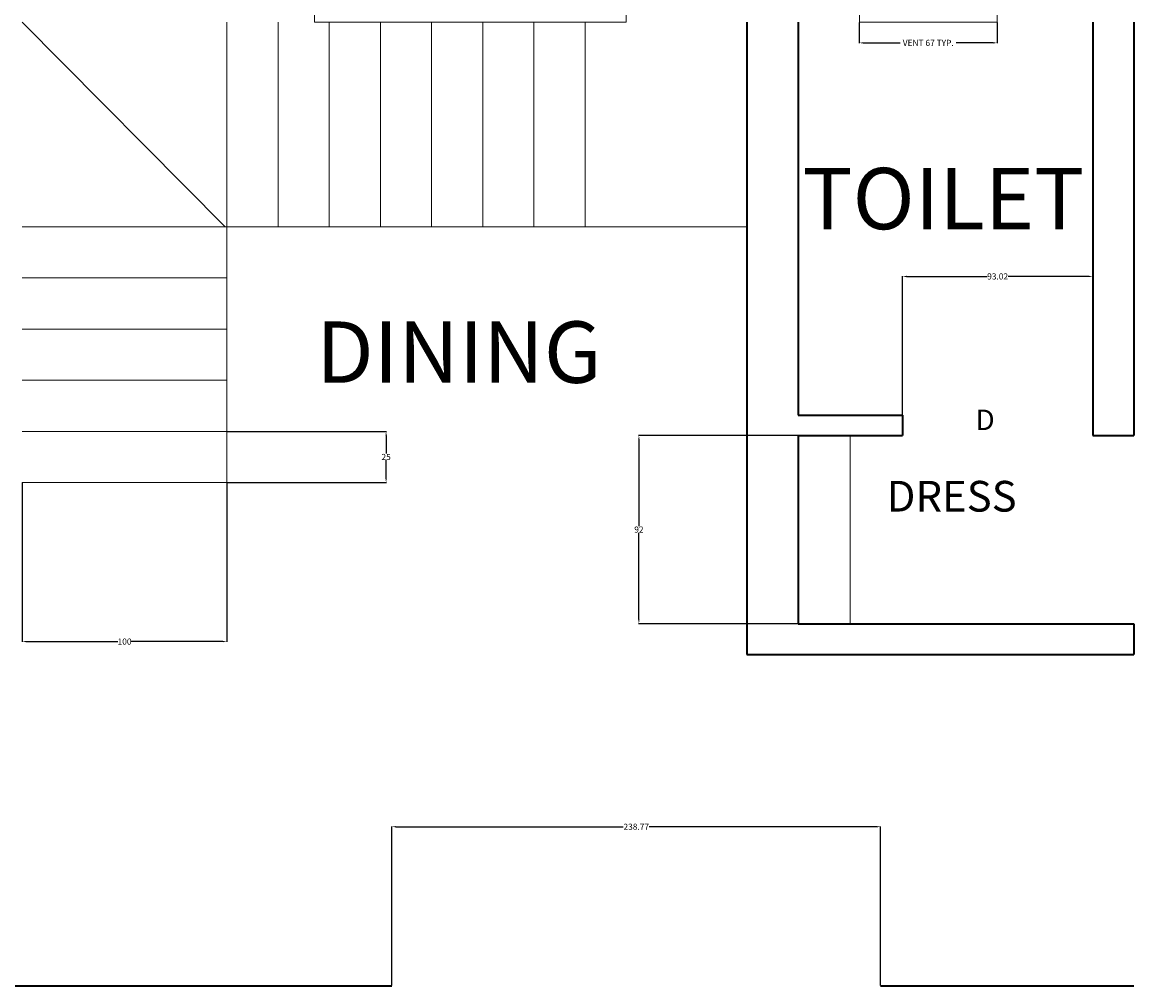
# Model space of a CAD drawing. Units: centimetres. Extents: x -121 to 3851, y -16 to 1180.
# Tile 5 of 16: x 415 to 958, y 384 to 855. Entities that reach past the tile are written whole.
import ezdxf

# ---------------------------------------------------------------- set-up
doc = ezdxf.new("R2010")
doc.units = ezdxf.units.CM
doc.header["$MEASUREMENT"] = 0
for name, color, linetype, lineweight in [('A-ANNO-DIMS', 2, 'Continuous', 18), ('A-ANNO-IDEN', 3, 'Continuous', 13), ('A-AREA-IDEN', 3, 'Continuous', 18), ('A-FLOR-CASE', 9, 'Continuous', 18), ('A-FLOR-STRS', 3, 'Continuous', 18), ('A-GLAZ', 4, 'Continuous', 18), ('A-WALL', 7, 'Continuous', 35)]:
    doc.layers.add(name, color=color, linetype=linetype, lineweight=lineweight)
doc.styles.get("Standard").update_dxf_attribs({"font": 'arial.ttf'})
doc.dimstyles.get("Standard").update_dxf_attribs({"dimtxt": 3, "dimasz": 2, "dimexe": 0.18, "dimexo": 0.0625, "dimgap": 0.09, "dimtad": 0, "dimtih": 1, "dimtoh": 1, "dimdec": 0, "dimzin": 0, "dimdsep": 46, "dimtxsty": 'Standard', "dimcen": 0.09, "dimadec": 0, "dimazin": 0, "dimtfac": 1, "dimtdec": 0, "dimtofl": 0, "dimtmove": 0, "dimatfit": 3, "dimfxl": 1, "dimtolj": 1, "dimtzin": 0, "dimarcsym": 0})

# ---------------------------------------------------------------- blocks, each defined once
blk = doc.blocks.new('WIN-152CM')
for p, q in [((0, 17.5), (152.19, 17.5)), ((0, 12.5), (152.19, 12.5)), ((0, 7.5), (152.19, 7.5))]:
    blk.add_line(p, q)
blk.add_lwpolyline([(0, 25), (152.19, 25), (152.19, 0), (0, 0)], close=True)
blk = doc.blocks.new('VENT-67CM')
for p, q in [((0, 15.5), (67.32, 15.5)), ((0, 12.5), (67.32, 12.5)), ((0, 9.5), (67.32, 9.5))]:
    blk.add_line(p, q)
blk.add_lwpolyline([(0, 25), (67.32, 25), (67.32, 0), (0, 0)], close=True)
blk = doc.blocks.new('STAIR-L-RETURN')
for p, q in [((0, 225), (99.13, 125)), ((100, 100), (100, 225)), ((125, 125), (125, 225)), ((150, 125), (150, 225)), ((175, 125), (175, 225)), ((200, 125), (200, 225)), ((225, 125), (225, 225)), ((250, 125), (250, 225)), ((275, 125), (275, 225)), ((0, 125), (99.13, 125)), ((99.13, 125), (354, 125)), ((100, 0), (100, 125)), ((0, 100), (100, 100)), ((0, 75), (100, 75)), ((0, 50), (100, 50)), ((0, 25), (100, 25)), ((0, 0), (100, 0))]:
    blk.add_line(p, q)
blk = doc.blocks.new('*D29')
at = {"layer": 'A-ANNO-DIMS', "color": 0, "lineweight": -2, "transparency": 16777216}
for p, q in [((823.97, 854.95), (823.97, 844.74)), ((891.29, 854.95), (891.29, 844.74)), ((825.97, 844.92), (843.99, 844.92)), ((889.29, 844.92), (871.27, 844.92))]:
    blk.add_line(p, q, dxfattribs=at)
at = {"layer": 'A-ANNO-DIMS', "color": 0, "transparency": 16777216}
for points in [[(825.97, 845.25), (825.97, 844.58), (823.97, 844.92)], [(889.29, 845.25), (889.29, 844.58), (891.29, 844.92)]]:
    blk.add_solid(points, dxfattribs=at)
at = {"layer": 'Defpoints', "color": 0, "transparency": 16777216}
for p in [(823.97, 855.01), (891.29, 855.01), (891.29, 844.92)]:
    blk.add_point(p, dxfattribs=at)
at = {"layer": 'A-ANNO-DIMS', "color": 0, "transparency": 16777216, "insert": (857.63, 844.92), "char_height": 3, "attachment_point": 5}
blk.add_mtext('\\A1;VENT 67 TYP.', dxfattribs=at)
blk = doc.blocks.new('*D45')
at = {"layer": 'A-ANNO-DIMS', "color": 0, "lineweight": -2, "transparency": 16777216}
for p, q in [((595.61, 384.08), (595.61, 461.94)), ((597.61, 461.76), (708.65, 461.76)), ((832.38, 461.76), (721.34, 461.76)), ((834.38, 384.08), (834.38, 461.94))]:
    blk.add_line(p, q, dxfattribs=at)
at = {"layer": 'A-ANNO-DIMS', "color": 0, "transparency": 16777216}
for points in [[(597.61, 462.1), (597.61, 461.43), (595.61, 461.76)], [(832.38, 462.1), (832.38, 461.43), (834.38, 461.76)]]:
    blk.add_solid(points, dxfattribs=at)
at = {"layer": 'Defpoints', "color": 0, "transparency": 16777216}
for p in [(834.38, 461.76), (595.61, 384.01), (834.38, 384.01)]:
    blk.add_point(p, dxfattribs=at)
at = {"layer": 'A-ANNO-DIMS', "color": 0, "transparency": 16777216, "insert": (715, 461.76), "char_height": 3, "attachment_point": 5}
blk.add_mtext('\\A1;238.77', dxfattribs=at)
blk = doc.blocks.new('*D56')
at = {"layer": 'A-ANNO-DIMS', "color": 0, "lineweight": -2, "transparency": 16777216}
for p, q in [((415.04, 629.95), (415.04, 552.08)), ((515.04, 629.95), (515.04, 552.08)), ((417.04, 552.26), (461.78, 552.26)), ((513.04, 552.26), (468.3, 552.26))]:
    blk.add_line(p, q, dxfattribs=at)
at = {"layer": 'A-ANNO-DIMS', "color": 0, "transparency": 16777216}
for points in [[(417.04, 552.6), (417.04, 551.93), (415.04, 552.26)], [(513.04, 552.6), (513.04, 551.93), (515.04, 552.26)]]:
    blk.add_solid(points, dxfattribs=at)
at = {"layer": 'Defpoints', "color": 0, "transparency": 16777216}
for p in [(415.04, 630.01), (515.04, 630.01), (415.04, 552.26)]:
    blk.add_point(p, dxfattribs=at)
at = {"layer": 'A-ANNO-DIMS', "color": 0, "transparency": 16777216, "insert": (465.04, 552.26), "char_height": 3, "attachment_point": 5}
blk.add_mtext('\\A1;100', dxfattribs=at)
blk = doc.blocks.new('*D57')
at = {"layer": 'A-ANNO-DIMS', "color": 0, "lineweight": -2, "transparency": 16777216}
for p, q in [((515.1, 655.01), (592.97, 655.01)), ((592.79, 653.01), (592.79, 644.14)), ((592.79, 632.01), (592.79, 640.89)), ((515.1, 630.01), (592.97, 630.01))]:
    blk.add_line(p, q, dxfattribs=at)
at = {"layer": 'A-ANNO-DIMS', "color": 0, "transparency": 16777216}
for points in [[(592.45, 653.01), (593.12, 653.01), (592.79, 655.01)], [(592.45, 632.01), (593.12, 632.01), (592.79, 630.01)]]:
    blk.add_solid(points, dxfattribs=at)
at = {"layer": 'Defpoints', "color": 0, "transparency": 16777216}
for p in [(515.04, 655.01), (515.04, 630.01), (592.79, 630.01)]:
    blk.add_point(p, dxfattribs=at)
at = {"layer": 'A-ANNO-DIMS', "color": 0, "transparency": 16777216, "insert": (592.79, 642.51), "char_height": 3, "attachment_point": 5}
blk.add_mtext('\\A1;25', dxfattribs=at)
blk = doc.blocks.new('*D58')
at = {"layer": 'A-ANNO-DIMS', "color": 0, "lineweight": -2, "transparency": 16777216}
for p, q in [((845.02, 653.08), (845.02, 730.94)), ((847.02, 730.76), (886.39, 730.76)), ((936.04, 730.76), (896.66, 730.76)), ((938.04, 653.08), (938.04, 730.94))]:
    blk.add_line(p, q, dxfattribs=at)
at = {"layer": 'A-ANNO-DIMS', "color": 0, "transparency": 16777216}
for points in [[(847.02, 731.1), (847.02, 730.43), (845.02, 730.76)], [(936.04, 731.1), (936.04, 730.43), (938.04, 730.76)]]:
    blk.add_solid(points, dxfattribs=at)
at = {"layer": 'Defpoints', "color": 0, "transparency": 16777216}
for p in [(938.04, 730.76), (845.02, 653.01), (938.04, 653.01)]:
    blk.add_point(p, dxfattribs=at)
at = {"layer": 'A-ANNO-DIMS', "color": 0, "transparency": 16777216, "insert": (891.53, 730.76), "char_height": 3, "attachment_point": 5}
blk.add_mtext('\\A1;93.02', dxfattribs=at)
blk = doc.blocks.new('*D59')
at = {"layer": 'A-ANNO-DIMS', "color": 0, "lineweight": -2, "transparency": 16777216}
for p, q in [((793.98, 653.01), (716.11, 653.01)), ((716.29, 651.01), (716.29, 608.64)), ((716.29, 563.01), (716.29, 605.39)), ((793.98, 561.01), (716.11, 561.01))]:
    blk.add_line(p, q, dxfattribs=at)
at = {"layer": 'A-ANNO-DIMS', "color": 0, "transparency": 16777216}
for points in [[(715.95, 651.01), (716.62, 651.01), (716.29, 653.01)], [(715.95, 563.01), (716.62, 563.01), (716.29, 561.01)]]:
    blk.add_solid(points, dxfattribs=at)
at = {"layer": 'Defpoints', "color": 0, "transparency": 16777216}
for p in [(716.29, 653.01), (794.04, 653.01), (794.04, 561.01)]:
    blk.add_point(p, dxfattribs=at)
at = {"layer": 'A-ANNO-DIMS', "color": 0, "transparency": 16777216, "insert": (716.29, 607.01), "char_height": 3, "attachment_point": 5}
blk.add_mtext('\\A1;92', dxfattribs=at)

msp = doc.modelspace()

# ---------------------------------------------------------------- linework, layer by layer
at = {"layer": 'A-FLOR-CASE'}
msp.add_line((819.5273, 653.0141), (819.5273, 561.0141), dxfattribs=at)
at = {"layer": 'A-WALL'}
for p, q in [((769.0382, 855.0141), (769.0382, 546.0141)), ((794.0382, 855.0141), (794.0382, 663.0141)), ((938.0382, 855.0141), (938.0382, 653.0141)), ((958.0382, 855.0141), (958.0382, 653.0141)), ((794.0382, 663.0141), (845.0164, 663.0141)), ((845.0164, 663.0141), (845.0164, 653.0141)), ((794.0382, 653.0141), (845.0164, 653.0141)), ((794.0382, 653.0141), (794.0382, 561.0141)), ((938.0382, 653.0141), (958.0382, 653.0141)), ((794.0382, 561.0141), (958.0382, 561.0141)), ((958.0382, 561.0141), (958.0382, 546.0141)), ((769.0382, 546.0141), (958.0382, 546.0141)), ((90.0382, 384.0141), (595.6084, 384.0141)), ((834.382, 384.0141), (958.0382, 384.0141))]:
    msp.add_line(p, q, dxfattribs=at)

# ---------------------------------------------------------------- block references
at = {"layer": 'A-FLOR-STRS'}
msp.add_blockref('STAIR-L-RETURN', (415.038, 630.014), dxfattribs=at)
at = {"layer": 'A-GLAZ'}
for name, p in [('WIN-152CM', (557.8305, 855.014)), ('VENT-67CM', (823.973, 855.014))]:
    msp.add_blockref(name, p, dxfattribs=at)

# ---------------------------------------------------------------- texts
at = {"layer": 'A-ANNO-IDEN', "insert": (880.7126, 665.6492), "char_height": 10, "attachment_point": 1}
msp.add_mtext_dynamic_manual_height_columns('D', width=55.718495, gutter_width=1, heights=[0], dxfattribs=at)
at = {"layer": 'A-AREA-IDEN', "attachment_point": 1}
for s, width, insert, char_height in [('TOILET', 114.065148, (796.1498, 783.8101), 30), ('DINING', 149.976594, (558.5678, 708.7424), 30), ('DRESS', 14.894434, (837.31, 630.808), 15)]:
    msp.add_mtext_dynamic_manual_height_columns(s, width=width, gutter_width=1, heights=[0], dxfattribs=dict(at, insert=insert, char_height=char_height))

# ---------------------------------------------------------------- dimensions: what is measured, and where the dimension line sits
at = {"layer": 'A-ANNO-DIMS'}
dim = msp.add_linear_dim(base=(891.2948, 844.9158), p1=(823.973, 855.0141), p2=(891.2948, 855.0141), text='VENT <> TYP.', dimstyle='Standard', override={"dimdec": 0, "dimlfac": 1, "dimrnd": 0, "dimzin": 0, "dimdsep": 46, "dimlunit": 2}, dxfattribs=at)
dim.commit()
dim.dimension.update_dxf_attribs({"geometry": '*D29', "text_midpoint": (857.6339, 844.9158)})
for base, p1, p2, picture, middle in [((938.0382, 730.7641), (845.0164, 653.0141), (938.0382, 653.0141), '*D58', (891.5273, 730.7641)), ((834.382, 461.7641), (595.6084, 384.0141), (834.382, 384.0141), '*D45', (714.9952, 461.7641))]:
    dim = msp.add_linear_dim(base=base, p1=p1, p2=p2, dimstyle='Standard', override={"dimdec": 2, "dimlfac": 1, "dimrnd": 0, "dimzin": 0, "dimdsep": 46, "dimlunit": 2}, dxfattribs=at)
    dim.commit()
    dim.dimension.update_dxf_attribs({"geometry": picture, "text_midpoint": middle})
for base, p1, p2, angle, picture, middle in [((592.7882, 630.0141), (515.0382, 655.0141), (515.0382, 630.0141), 270, '*D57', (592.7882, 642.5141)), ((716.2882, 653.0141), (794.0382, 561.0141), (794.0382, 653.0141), 90, '*D59', (716.2882, 607.0141)), ((415.0382, 552.2641), (515.0382, 630.0141), (415.0382, 630.0141), 180, '*D56', (465.0382, 552.2641))]:
    dim = msp.add_linear_dim(base=base, p1=p1, p2=p2, angle=angle, dimstyle='Standard', override={"dimdec": 0, "dimlfac": 1, "dimrnd": 0, "dimzin": 0, "dimdsep": 46, "dimlunit": 2}, dxfattribs=at)
    dim.commit()
    dim.dimension.update_dxf_attribs({"geometry": picture, "text_midpoint": middle})

doc.saveas('drawing.dxf')
